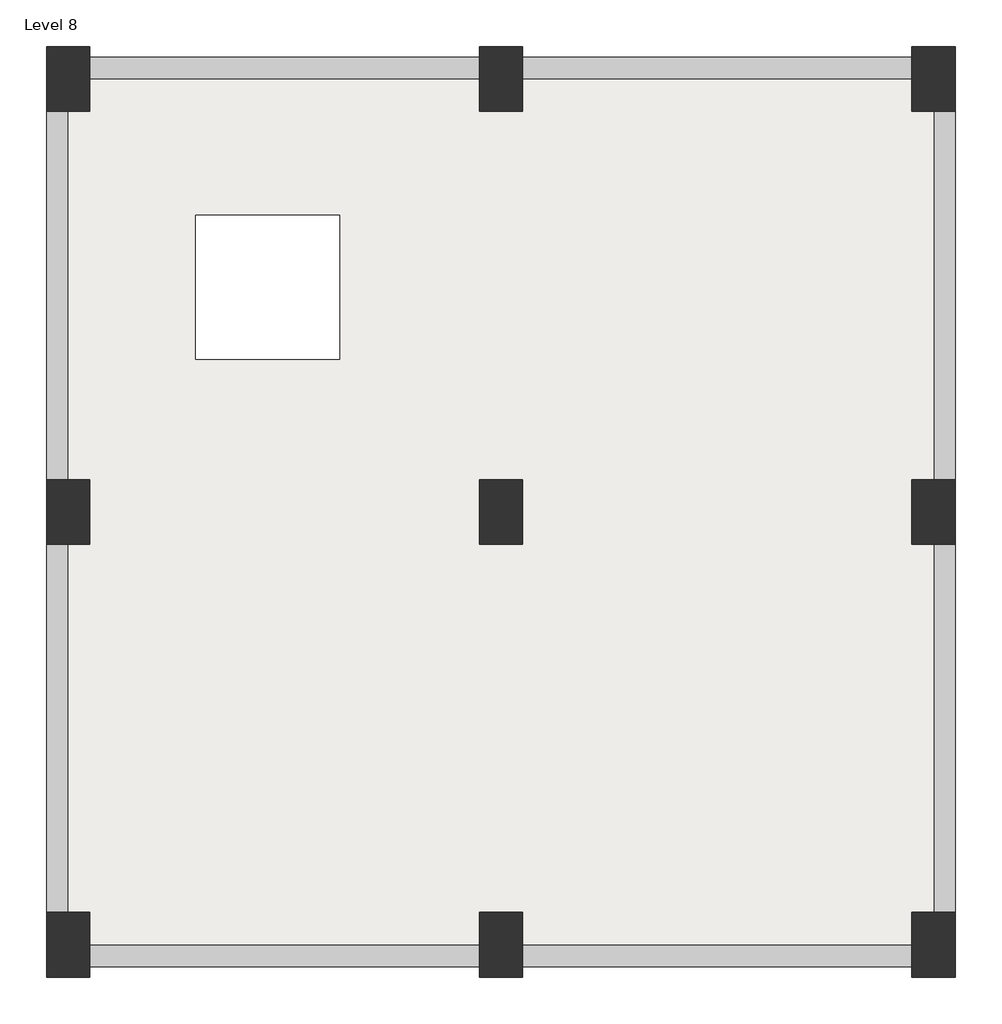
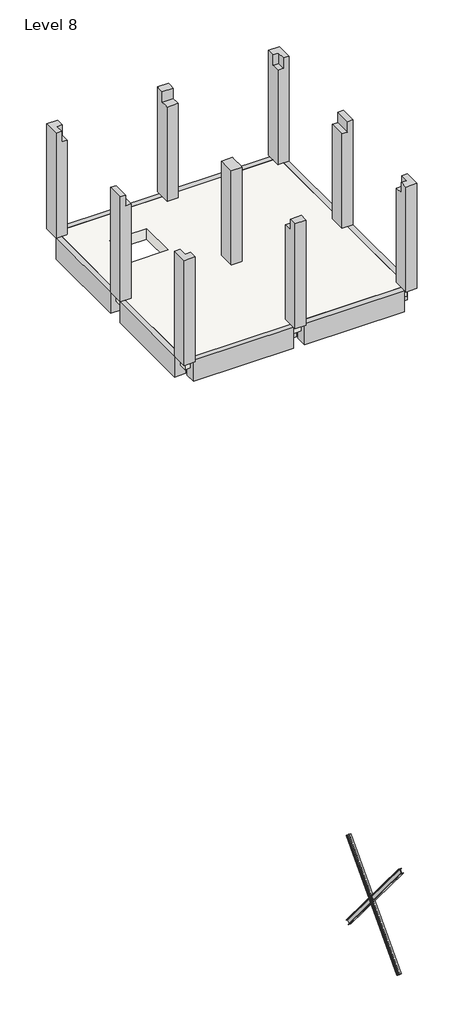
# One storey: 9 columns, 6 beams, 2 members, 1 slab.
"""IFC4 building model written with IfcOpenShell, lengths in millimetres."""

from ifc_helpers import new_model, si_unit, frame, origin, place, context, project, spatial, polyline, outline, extrude, faceted_brep, transform, mapped, element, save
from components import ub_universal_beams_ub127x76x13_5fda7735, ub_universal_beams_ub127x76x13_96cbbb94

model = new_model("IFC4")

# Units and contexts
model_context = context("Model", 3, world=origin())
ifc_project = project(units=[si_unit("LENGTHUNIT", "METRE", prefix="MILLI")], contexts=[model_context])

# Site, building, storey
site = spatial("IfcSite", under=ifc_project)
building = spatial("IfcBuilding", under=site)
storey = spatial("IfcBuildingStorey", under=building, Name="Level 8", Elevation=21000.0)

# Beams
placement = place(None, origin())
element("IfcBeam", 1, ObjectType="Concrete-Rectangular Beam : 300 x 600mm", at=placement, inside=storey, context=model_context, shape_type="SweptSolid", body=[
    extrude(outline(polyline([(526.3372902, 20400.0), (226.3372902, 20400.0), (226.3372902, 20700.0), (376.3372902, 20700.0), (376.3372902, 21000.0), (526.3372902, 21000.0), (526.3372902, 20400.0)])), frame((2068.7595868, 0.0, 0.0), z_axis=(1.0, 0.0, 0.0), x_axis=(0.0, 1.0, 0.0)), (0.0, 0.0, 1.0), 2700.0),
    extrude(outline(polyline([(526.3372902, 20400.0), (226.3372902, 20400.0), (226.3372902, 20700.0), (376.3372902, 20700.0), (376.3372902, 21000.0), (526.3372902, 21000.0), (526.3372902, 20400.0)])), frame((-931.2404132, 0.0, 0.0), z_axis=(1.0, 0.0, 0.0), x_axis=(0.0, 1.0, 0.0)), (0.0, 0.0, 1.0), 2700.0),
])
element("IfcBeam", 2, ObjectType="Concrete-Rectangular Beam : 300 x 600mm", at=placement, inside=storey, context=model_context, shape_type="SweptSolid", body=[
    extrude(outline(polyline([(20400.0, 5068.7595868), (21000.0, 5068.7595868), (21000.0, 4918.7595868), (20700.0, 4918.7595868), (20700.0, 4768.7595868), (20400.0, 4768.7595868), (20400.0, 5068.7595868)])), frame((0.0, -2398.6627098, 0.0), z_axis=(0.0, 1.0, 0.0), x_axis=(0.0, 0.0, 1.0)), (0.0, 0.0, 1.0), 2550.0),
    extrude(outline(polyline([(20400.0, 5068.7595868), (21000.0, 5068.7595868), (21000.0, 4918.7595868), (20700.0, 4918.7595868), (20700.0, 4768.7595868), (20400.0, 4768.7595868), (20400.0, 5068.7595868)])), frame((0.0, -5398.6627098, 0.0), z_axis=(0.0, 1.0, 0.0), x_axis=(0.0, 0.0, 1.0)), (0.0, 0.0, 1.0), 2550.0),
])
element("IfcBeam", 3, ObjectType="Concrete-Rectangular Beam : 300 x 600mm", at=placement, inside=storey, context=model_context, shape_type="SweptSolid", body=[
    extrude(outline(polyline([(-5773.6627098, 20400.0), (-5773.6627098, 21000.0), (-5623.6627098, 21000.0), (-5623.6627098, 20700.0), (-5473.6627098, 20700.0), (-5473.6627098, 20400.0), (-5773.6627098, 20400.0)])), frame((2068.7595868, 0.0, 0.0), z_axis=(1.0, 0.0, 0.0), x_axis=(0.0, 1.0, 0.0)), (0.0, 0.0, 1.0), 2700.0),
    extrude(outline(polyline([(-5773.6627098, 20400.0), (-5773.6627098, 21000.0), (-5623.6627098, 21000.0), (-5623.6627098, 20700.0), (-5473.6627098, 20700.0), (-5473.6627098, 20400.0), (-5773.6627098, 20400.0)])), frame((-931.2404132, 0.0, 0.0), z_axis=(1.0, 0.0, 0.0), x_axis=(0.0, 1.0, 0.0)), (0.0, 0.0, 1.0), 2700.0),
])
element("IfcBeam", 4, ObjectType="Concrete-Rectangular Beam : 300 x 600mm", at=placement, inside=storey, context=model_context, shape_type="SweptSolid", body=[
    extrude(outline(polyline([(21000.0, -1231.2404132), (20400.0, -1231.2404132), (20400.0, -931.2404132), (20700.0, -931.2404132), (20700.0, -1081.2404132), (21000.0, -1081.2404132), (21000.0, -1231.2404132)])), frame((0.0, -5398.6627098, 0.0), z_axis=(0.0, 1.0, 0.0), x_axis=(0.0, 0.0, 1.0)), (0.0, 0.0, 1.0), 2550.0),
    extrude(outline(polyline([(21000.0, -1231.2404132), (20400.0, -1231.2404132), (20400.0, -931.2404132), (20700.0, -931.2404132), (20700.0, -1081.2404132), (21000.0, -1081.2404132), (21000.0, -1231.2404132)])), frame((0.0, -2398.6627098, 0.0), z_axis=(0.0, 1.0, 0.0), x_axis=(0.0, 0.0, 1.0)), (0.0, 0.0, 1.0), 2550.0),
])
element("IfcBeam", 5, ObjectType="Concrete-Rectangular Beam : 300 x 600mm", at=placement, inside=storey, context=model_context, shape_type="SweptSolid", body=[
    extrude(outline(polyline([(2068.7595868, -5398.6627098), (1768.7595868, -5398.6627098), (1768.7595868, -2848.6627098), (2068.7595868, -2848.6627098), (2068.7595868, -5398.6627098)])), frame((0.0, 0.0, 20400.0), z_axis=(0.0, 0.0, 1.0), x_axis=(1.0, 0.0, 0.0)), (0.0, 0.0, 1.0), 300.0),
    extrude(outline(polyline([(1768.7595868, 151.3372902), (2068.7595868, 151.3372902), (2068.7595868, -2398.6627098), (1768.7595868, -2398.6627098), (1768.7595868, 151.3372902)])), frame((0.0, 0.0, 20400.0), z_axis=(0.0, 0.0, 1.0), x_axis=(1.0, 0.0, 0.0)), (0.0, 0.0, 1.0), 300.0),
])
element("IfcBeam", 6, ObjectType="Concrete-Rectangular Beam : 300 x 600mm", at=placement, inside=storey, context=model_context, shape_type="SweptSolid", body=[
    extrude(outline(polyline([(4768.7595868, -2473.6627098), (4768.7595868, -2773.6627098), (2068.7595868, -2773.6627098), (2068.7595868, -2473.6627098), (4768.7595868, -2473.6627098)])), frame((0.0, 0.0, 20400.0), z_axis=(0.0, 0.0, 1.0), x_axis=(1.0, 0.0, 0.0)), (0.0, 0.0, 1.0), 300.0),
    extrude(outline(polyline([(-931.2404132, -2773.6627098), (-931.2404132, -2473.6627098), (1768.7595868, -2473.6627098), (1768.7595868, -2773.6627098), (-931.2404132, -2773.6627098)])), frame((0.0, 0.0, 20400.0), z_axis=(0.0, 0.0, 1.0), x_axis=(1.0, 0.0, 0.0)), (0.0, 0.0, 1.0), 300.0),
])

# Columns
element("IfcColumn", 7, ObjectType="Concrete-Rectangular-Column : 300 x 450mm", at=placement, inside=storey, context=model_context, shape_type="Brep", body=[
    faceted_brep([(-1231.2404132, -5848.6627098, 24000.0), (-931.2404132, -5848.6627098, 24000.0), (-931.2404132, -5623.6627098, 24000.0), (-1081.2404132, -5623.6627098, 24000.0), (-1081.2404132, -5398.6627098, 24000.0), (-1231.2404132, -5398.6627098, 24000.0), (-1231.2404132, -5848.6627098, 21000.0), (-1231.2404132, -5398.6627098, 21000.0), (-931.2404132, -5398.6627098, 21000.0), (-931.2404132, -5848.6627098, 21000.0), (-931.2404132, -5398.6627098, 23700.0), (-931.2404132, -5623.6627098, 23700.0), (-1081.2404132, -5398.6627098, 23700.0), (-1081.2404132, -5623.6627098, 23700.0)], [[[0, 1, 2, 3, 4, 5]], [[6, 7, 8, 9]], [[1, 0, 6, 9]], [[9, 8, 10, 11, 2, 1]], [[8, 7, 5, 4, 12, 10]], [[0, 5, 7, 6]], [[12, 13, 11, 10]], [[13, 3, 2, 11]], [[3, 13, 12, 4]]]),
])
element("IfcColumn", 8, ObjectType="Concrete-Rectangular-Column : 300 x 450mm", at=placement, inside=storey, context=model_context, shape_type="Brep", body=[
    faceted_brep([(1768.7595868, -5848.6627098, 24000.0), (2068.7595868, -5848.6627098, 24000.0), (2068.7595868, -5773.6627098, 24000.0), (2068.7595868, -5623.6627098, 24000.0), (1768.7595868, -5623.6627098, 24000.0), (1768.7595868, -5773.6627098, 24000.0), (1768.7595868, -5848.6627098, 21000.0), (1768.7595868, -5398.6627098, 21000.0), (2068.7595868, -5398.6627098, 21000.0), (2068.7595868, -5848.6627098, 21000.0), (2068.7595868, -5398.6627098, 23700.0), (2068.7595868, -5473.6627098, 23700.0), (2068.7595868, -5623.6627098, 23700.0), (1768.7595868, -5398.6627098, 23700.0), (1768.7595868, -5623.6627098, 23700.0), (1768.7595868, -5473.6627098, 23700.0)], [[[0, 1, 2, 3, 4, 5]], [[6, 7, 8, 9]], [[1, 0, 6, 9]], [[9, 8, 10, 11, 12, 3, 2, 1]], [[8, 7, 13, 10]], [[7, 6, 0, 5, 4, 14, 15, 13]], [[14, 12, 11, 10, 13, 15]], [[12, 14, 4, 3]]]),
])
element("IfcColumn", 9, ObjectType="Concrete-Rectangular-Column : 300 x 450mm", at=placement, inside=storey, context=model_context, shape_type="Brep", body=[
    faceted_brep([(4768.7595868, -5848.6627098, 24000.0), (5068.7595868, -5848.6627098, 24000.0), (5068.7595868, -5398.6627098, 24000.0), (4918.7595868, -5398.6627098, 24000.0), (4918.7595868, -5623.6627098, 24000.0), (4768.7595868, -5623.6627098, 24000.0), (4768.7595868, -5848.6627098, 21000.0), (4768.7595868, -5398.6627098, 21000.0), (5068.7595868, -5398.6627098, 21000.0), (5068.7595868, -5848.6627098, 21000.0), (4768.7595868, -5398.6627098, 23700.0), (4918.7595868, -5398.6627098, 23700.0), (4768.7595868, -5623.6627098, 23700.0), (4918.7595868, -5623.6627098, 23700.0)], [[[0, 1, 2, 3, 4, 5]], [[6, 7, 8, 9]], [[1, 0, 6, 9]], [[2, 1, 9, 8]], [[8, 7, 10, 11, 3, 2]], [[7, 6, 0, 5, 12, 10]], [[12, 13, 11, 10]], [[13, 4, 3, 11]], [[4, 13, 12, 5]]]),
])
element("IfcColumn", 10, ObjectType="Concrete-Rectangular-Column : 300 x 450mm", at=placement, inside=storey, context=model_context, shape_type="Brep", body=[
    faceted_brep([(-1231.2404132, -2398.6627098, 24000.0), (-1231.2404132, -2848.6627098, 24000.0), (-1081.2404132, -2848.6627098, 24000.0), (-1081.2404132, -2398.6627098, 24000.0), (-1231.2404132, -2848.6627098, 21000.0), (-1231.2404132, -2398.6627098, 21000.0), (-931.2404132, -2398.6627098, 21000.0), (-931.2404132, -2848.6627098, 21000.0), (-931.2404132, -2848.6627098, 23400.0), (-931.2404132, -2848.6627098, 23700.0), (-1081.2404132, -2848.6627098, 23700.0), (-1231.2404132, -2848.6627098, 23400.0), (-931.2404132, -2398.6627098, 23400.0), (-931.2404132, -2398.6627098, 23700.0), (-1231.2404132, -2398.6627098, 23400.0), (-1081.2404132, -2398.6627098, 23700.0)], [[[0, 1, 2, 3]], [[4, 5, 6, 7]], [[4, 7, 8, 9, 10, 2, 1, 11]], [[7, 6, 12, 13, 9, 8]], [[6, 5, 14, 0, 3, 15, 13, 12]], [[1, 0, 14, 5, 4, 11]], [[15, 10, 9, 13]], [[10, 15, 3, 2]]]),
])
element("IfcColumn", 11, ObjectType="Concrete-Rectangular-Column : 300 x 450mm", at=placement, inside=storey, context=model_context, shape_type="Brep", body=[
    faceted_brep([(1768.7595868, -2848.6627098, 21000.0), (1768.7595868, -2398.6627098, 21000.0), (2068.7595868, -2398.6627098, 21000.0), (2068.7595868, -2848.6627098, 21000.0), (2068.7595868, -2848.6627098, 23400.0), (2068.7595868, -2848.6627098, 23700.0), (1768.7595868, -2848.6627098, 23700.0), (1768.7595868, -2848.6627098, 23400.0), (2068.7595868, -2398.6627098, 23400.0), (2068.7595868, -2398.6627098, 23700.0), (2068.7595868, -2473.6627098, 23700.0), (2068.7595868, -2773.6627098, 23700.0), (1768.7595868, -2398.6627098, 23400.0), (1768.7595868, -2398.6627098, 23700.0), (1768.7595868, -2773.6627098, 23700.0), (1768.7595868, -2473.6627098, 23700.0)], [[[0, 1, 2, 3]], [[0, 3, 4, 5, 6, 7]], [[3, 2, 8, 9, 10, 11, 5, 4]], [[2, 1, 12, 13, 9, 8]], [[1, 0, 7, 6, 14, 15, 13, 12]], [[6, 5, 11, 10, 9, 13, 15, 14]]]),
])
element("IfcColumn", 12, ObjectType="Concrete-Rectangular-Column : 300 x 450mm", at=placement, inside=storey, context=model_context, shape_type="Brep", body=[
    faceted_brep([(5068.7595868, -2848.6627098, 24000.0), (5068.7595868, -2398.6627098, 24000.0), (4918.7595868, -2398.6627098, 24000.0), (4918.7595868, -2848.6627098, 24000.0), (4768.7595868, -2848.6627098, 21000.0), (4768.7595868, -2398.6627098, 21000.0), (5068.7595868, -2398.6627098, 21000.0), (5068.7595868, -2848.6627098, 21000.0), (5068.7595868, -2848.6627098, 23400.0), (4918.7595868, -2848.6627098, 23700.0), (4768.7595868, -2848.6627098, 23700.0), (4768.7595868, -2848.6627098, 23400.0), (5068.7595868, -2398.6627098, 23400.0), (4768.7595868, -2398.6627098, 23400.0), (4768.7595868, -2398.6627098, 23700.0), (4918.7595868, -2398.6627098, 23700.0)], [[[0, 1, 2, 3]], [[4, 5, 6, 7]], [[4, 7, 8, 0, 3, 9, 10, 11]], [[1, 0, 8, 7, 6, 12]], [[6, 5, 13, 14, 15, 2, 1, 12]], [[5, 4, 11, 10, 14, 13]], [[9, 15, 14, 10]], [[15, 9, 3, 2]]]),
])
element("IfcColumn", 13, ObjectType="Concrete-Rectangular-Column : 300 x 450mm", at=placement, inside=storey, context=model_context, shape_type="Brep", body=[
    faceted_brep([(-931.2404132, 601.3372902, 24000.0), (-1231.2404132, 601.3372902, 24000.0), (-1231.2404132, 151.3372902, 24000.0), (-1081.2404132, 151.3372902, 24000.0), (-1081.2404132, 376.3372902, 24000.0), (-931.2404132, 376.3372902, 24000.0), (-1231.2404132, 151.3372902, 21000.0), (-1231.2404132, 601.3372902, 21000.0), (-931.2404132, 601.3372902, 21000.0), (-931.2404132, 151.3372902, 21000.0), (-931.2404132, 151.3372902, 23700.0), (-1081.2404132, 151.3372902, 23700.0), (-931.2404132, 376.3372902, 23700.0), (-1081.2404132, 376.3372902, 23700.0)], [[[0, 1, 2, 3, 4, 5]], [[6, 7, 8, 9]], [[6, 9, 10, 11, 3, 2]], [[9, 8, 0, 5, 12, 10]], [[1, 0, 8, 7]], [[2, 1, 7, 6]], [[12, 13, 11, 10]], [[13, 4, 3, 11]], [[4, 13, 12, 5]]]),
])
element("IfcColumn", 14, ObjectType="Concrete-Rectangular-Column : 300 x 450mm", at=placement, inside=storey, context=model_context, shape_type="Brep", body=[
    faceted_brep([(2068.7595868, 601.3372902, 24000.0), (1768.7595868, 601.3372902, 24000.0), (1768.7595868, 526.3372902, 24000.0), (1768.7595868, 376.3372902, 24000.0), (2068.7595868, 376.3372902, 24000.0), (2068.7595868, 526.3372902, 24000.0), (1768.7595868, 151.3372902, 21000.0), (1768.7595868, 601.3372902, 21000.0), (2068.7595868, 601.3372902, 21000.0), (2068.7595868, 151.3372902, 21000.0), (2068.7595868, 151.3372902, 23700.0), (1768.7595868, 151.3372902, 23700.0), (2068.7595868, 376.3372902, 23700.0), (2068.7595868, 226.3372902, 23700.0), (1768.7595868, 226.3372902, 23700.0), (1768.7595868, 376.3372902, 23700.0)], [[[0, 1, 2, 3, 4, 5]], [[6, 7, 8, 9]], [[6, 9, 10, 11]], [[9, 8, 0, 5, 4, 12, 13, 10]], [[1, 0, 8, 7]], [[7, 6, 11, 14, 15, 3, 2, 1]], [[12, 15, 14, 11, 10, 13]], [[15, 12, 4, 3]]]),
])
element("IfcColumn", 15, ObjectType="Concrete-Rectangular-Column : 300 x 450mm", at=placement, inside=storey, context=model_context, shape_type="Brep", body=[
    faceted_brep([(5068.7595868, 151.3372902, 24000.0), (5068.7595868, 601.3372902, 24000.0), (4768.7595868, 601.3372902, 24000.0), (4768.7595868, 376.3372902, 24000.0), (4918.7595868, 376.3372902, 24000.0), (4918.7595868, 151.3372902, 24000.0), (4768.7595868, 151.3372902, 21000.0), (4768.7595868, 601.3372902, 21000.0), (5068.7595868, 601.3372902, 21000.0), (5068.7595868, 151.3372902, 21000.0), (4918.7595868, 151.3372902, 23700.0), (4768.7595868, 151.3372902, 23700.0), (4768.7595868, 376.3372902, 23700.0), (4918.7595868, 376.3372902, 23700.0)], [[[0, 1, 2, 3, 4, 5]], [[6, 7, 8, 9]], [[6, 9, 0, 5, 10, 11]], [[1, 0, 9, 8]], [[2, 1, 8, 7]], [[7, 6, 11, 12, 3, 2]], [[13, 12, 11, 10]], [[4, 13, 10, 5]], [[13, 4, 3, 12]]]),
])

# Members
ub_universal_beams_ub127x76x13_shape = ub_universal_beams_ub127x76x13_5fda7735(model_context)
element("IfcMember", 16, ObjectType="UB-Universal Beams : UB127x76x13", at=placement, inside=storey, context=model_context, shape_type="MappedRepresentation", body=[
    mapped(ub_universal_beams_ub127x76x13_shape, transform((4918.7595868, -3987.3365723, 2466.3104182), x_axis=(0.0, 0.6408125760238288, -0.7676973638157842), y_axis=(-1.0, 0.0, 0.0), z_axis=(0.0, 0.7676973638157842, 0.6408125760238288))),
])
ub_universal_beams_ub127x76x13_2_shape = ub_universal_beams_ub127x76x13_96cbbb94(model_context)
element("IfcMember", 17, ObjectType="UB-Universal Beams : UB127x76x13", at=placement, inside=storey, context=model_context, shape_type="MappedRepresentation", body=[
    mapped(ub_universal_beams_ub127x76x13_2_shape, transform((4918.7595868, -3946.516498, 2534.1249429), x_axis=(0.0, -0.6780160909774431, -0.7350470599734874), y_axis=(1.0, 0.0, 0.0), z_axis=(0.0, -0.7350470599734874, 0.6780160909774431))),
])

# Slab
element("IfcSlab", 18, ObjectType="Generic 300mm", at=placement, inside=storey, context=model_context, shape_type="Brep", body=[
    faceted_brep([(4918.7595868, 376.3372902, 20700.0), (4918.7595868, 151.3372902, 20700.0), (4918.7595868, -2398.6627098, 20700.0), (4918.7595868, -2848.6627098, 20700.0), (4918.7595868, -5398.6627098, 20700.0), (4918.7595868, -5623.6627098, 20700.0), (4768.7595868, -5623.6627098, 20700.0), (2068.7595868, -5623.6627098, 20700.0), (1768.7595868, -5623.6627098, 20700.0), (-931.2404132, -5623.6627098, 20700.0), (-1081.2404132, -5623.6627098, 20700.0), (-1081.2404132, -5398.6627098, 20700.0), (-1081.2404132, -2848.6627098, 20700.0), (-1081.2404132, -2398.6627098, 20700.0), (-1081.2404132, 151.3372902, 20700.0), (-1081.2404132, 376.3372902, 20700.0), (-931.2404132, 376.3372902, 20700.0), (1768.7595868, 376.3372902, 20700.0), (2068.7595868, 376.3372902, 20700.0), (4768.7595868, 376.3372902, 20700.0), (-198.5229478, -1566.5574371, 20700.0), (801.4770522, -1566.5574371, 20700.0), (801.4770522, -566.5574371, 20700.0), (-198.5229478, -566.5574371, 20700.0), (4918.7595868, -5623.6627098, 21000.0), (4918.7595868, -5398.6627098, 21000.0), (4918.7595868, -2848.6627098, 21000.0), (4918.7595868, -2398.6627098, 21000.0), (4918.7595868, 151.3372902, 21000.0), (4918.7595868, 376.3372902, 21000.0), (4768.7595868, 376.3372902, 21000.0), (2068.7595868, 376.3372902, 21000.0), (1768.7595868, 376.3372902, 21000.0), (-931.2404132, 376.3372902, 21000.0), (-1081.2404132, 376.3372902, 21000.0), (-1081.2404132, 151.3372902, 21000.0), (-1081.2404132, -2398.6627098, 21000.0), (-1081.2404132, -2848.6627098, 21000.0), (-1081.2404132, -5398.6627098, 21000.0), (-1081.2404132, -5623.6627098, 21000.0), (-931.2404132, -5623.6627098, 21000.0), (1768.7595868, -5623.6627098, 21000.0), (2068.7595868, -5623.6627098, 21000.0), (4768.7595868, -5623.6627098, 21000.0), (801.4770522, -1566.5574371, 21000.0), (-198.5229478, -1566.5574371, 21000.0), (-198.5229478, -566.5574371, 21000.0), (801.4770522, -566.5574371, 21000.0)], [[[0, 1, 2, 3, 4, 5, 6, 7, 8, 9, 10, 11, 12, 13, 14, 15, 16, 17, 18, 19], [20, 21, 22, 23]], [[24, 25, 26, 27, 28, 29, 30, 31, 32, 33, 34, 35, 36, 37, 38, 39, 40, 41, 42, 43], [44, 45, 46, 47]], [[5, 4, 3, 2, 1, 0, 29, 28, 27, 26, 25, 24]], [[10, 9, 8, 7, 6, 5, 24, 43, 42, 41, 40, 39]], [[15, 14, 13, 12, 11, 10, 39, 38, 37, 36, 35, 34]], [[0, 19, 18, 17, 16, 15, 34, 33, 32, 31, 30, 29]], [[20, 45, 44, 21]], [[21, 44, 47, 22]], [[22, 47, 46, 23]], [[45, 20, 23, 46]]]),
])

save(model, "model.ifc")

# Revit data of these elements
# Type "Concrete-Rectangular Beam : 300 x 600mm"
#   Length [instance default] = 1.524 m
#   b = 0.3 m
#   h = 0.6 m
#   Structural Material [instance default] = Concrete, Cast-in-Place gray
#   Assembly Code = ""
# Type "Concrete-Rectangular-Column : 300 x 450mm"
#   b = 0.3 m
#   h = 0.45 m
#   Structural Material [instance default] = Concrete, Cast-in-Place gray
# Type "UB-Universal Beams : UB127x76x13"
#   Section Name Key = "UB127X76X13"
#   Width = 7.6 cm
#   Web Thickness = 0.4 cm
#   Web Fillet = 0.76 cm
#   Warping Constant = 2000.0 cm⁶
#   Torsional Moment of Inertia = 2.85 cm⁴
#   Section Area = 16.5 cm²
#   Plastic Modulus weak axis = 22.6 cm³
#   Plastic Modulus strong axis = 84.2 cm³
#   Nominal Weight = 13.00 kgf/m
#   Moment of Inertia weak axis = 55.70 cm⁴
#   Moment of Inertia strong axis = 473.00 cm⁴
#   Height = 12.7 cm
#   Flange Thickness = 0.76 cm
#   Elastic Modulus weak axis = 14.7 cm³
#   Elastic Modulus strong axis = 74.6 cm³
#   Centroid Vertical = 6.35 cm
#   Centroid Horizontal = 3.8 cm
#   Bolt Spacing = 4.0 cm
#   Length [instance default] = 1.5 m
#   Structural Material [instance default] = Metal - Steel 43-275
#   Type Comments = ""
#   Assembly Code = ""
# Type "Generic 300mm"
#   Function = 0
#   Layers, outside or top first: 0.3 m no material (function 1)
# Elements 1, 2, 3, 4, 5, 6 (IfcBeam, "Concrete-Rectangular Beam : 300 x 600mm")
#   Structural Material = Concrete, Cast-in-Place gray
#   Phase Created = New Construction
#   Materials on its faces: "Concrete, Cast-in-Place gray"
# Elements 7, 8, 9, 10, 11, 12, 13, 14, 15 (IfcColumn, "Concrete-Rectangular-Column : 300 x 450mm")
#   Structural Material = Concrete, Cast-in-Place gray
#   Phase Created = New Construction
#   Materials on its faces: "Concrete, Cast-in-Place gray"
# Elements 16, 17 (IfcMember, "UB-Universal Beams : UB127x76x13")
#   Structural Material = Metal - Steel 43-275
#   Phase Created = New Construction
#   Materials on its faces: "Metal - Steel 43-275"
# Element 18 (IfcSlab, "Generic 300mm")
#   Height Offset From Level = 0 m
#   built-in parameter 1001954 = 1
#   Phase Created = New Construction
#   Materials on its faces: "Default Floor"
# Materials
#   "Concrete, Cast-in-Place gray": class "Concrete", colour RGB 192 192 192, transparency 0, Description = "Cast-in-place concrete", Cost = 0
#   "Metal - Steel 43-275": class "Metal", colour RGB 247 247 247, transparency 0, Cost = 0
#   "Default Floor": colour RGB 127 127 127, transparency 0, Cost = 0
